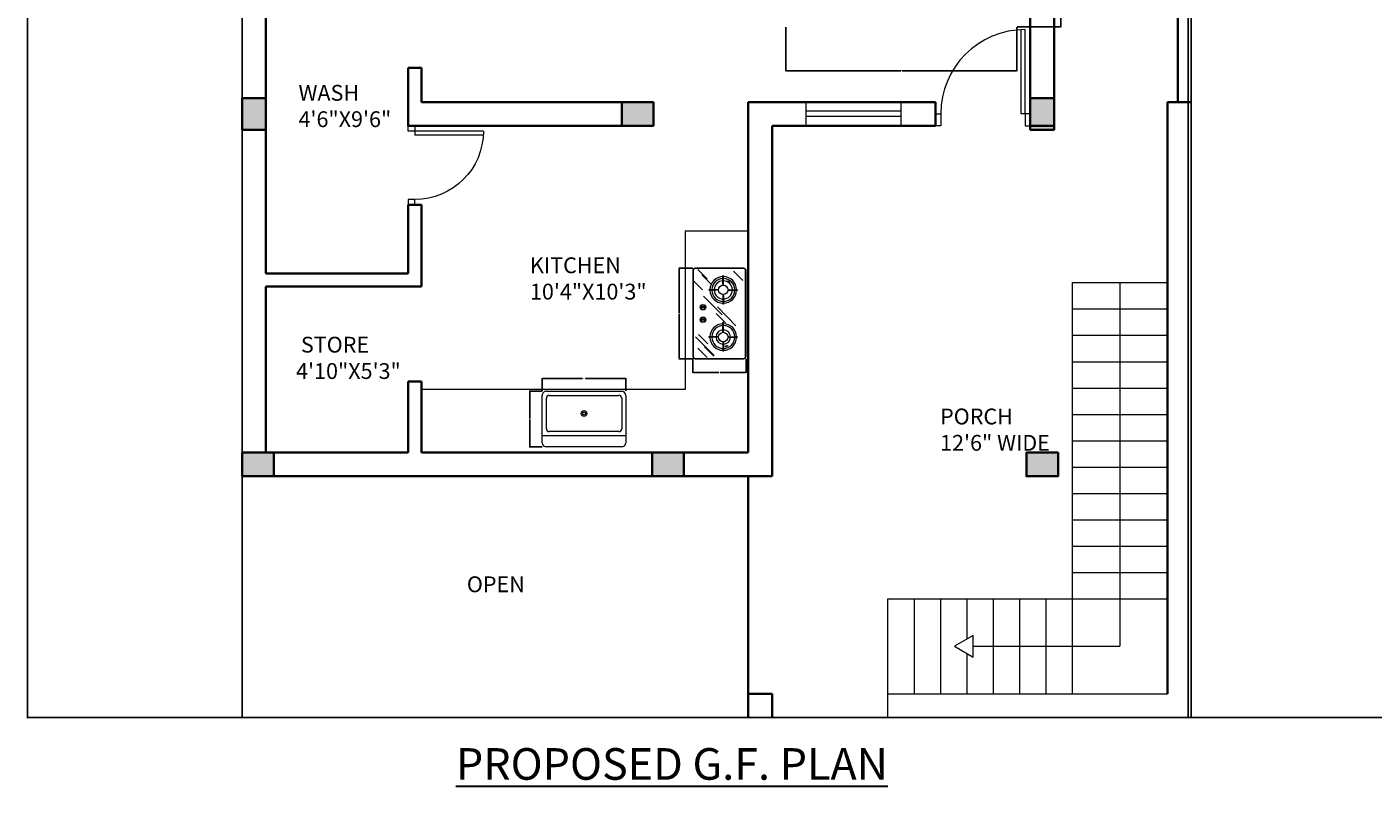
# Model space of a CAD drawing. Units: inches. Extents: x 1602 to 2642, y 1463 to 2270.
# Tile 1 of 5: x 1602 to 2113, y 1475 to 1763. Entities that reach past the tile are written whole.
import ezdxf

# ---------------------------------------------------------------- set-up
doc = ezdxf.new("R2010")
doc.units = ezdxf.units.IN
for name, color, linetype, lineweight in [('A-ANNO-DIMS', 2, 'Continuous', 18), ('A-ANNO-TEXT', 7, 'Continuous', 30), ('A-AREA-IDEN', 7, 'Continuous', 18), ('A-COLS', 7, 'Continuous', 35), ('A-DOOR', 3, 'Continuous', 18), ('A-EQPM', 8, 'Continuous', 18), ('A-FLOR-CASE', 9, 'Continuous', 18), ('A-FLOR-FIXT', 8, 'Continuous', 18), ('A-FLOR-STRS', 7, 'Continuous', 18), ('A-GLAZ', 4, 'Continuous', 18), ('A-WALL', 7, 'Continuous', 35), ('C-PROP', 7, 'Continuous', 25)]:
    doc.layers.add(name, color=color, linetype=linetype, lineweight=lineweight)
doc.styles.add('ATTR', font='romans.shx', dxfattribs={"width": 0.8, "height": 1.075})
doc.styles.get("Standard").update_dxf_attribs({"font": 'arial.ttf'})
doc.dimstyles.get("Standard").update_dxf_attribs({"dimtxt": 0.18, "dimasz": 0.18, "dimexe": 0.18, "dimexo": 0.0625, "dimgap": 0.09, "dimtad": 0, "dimtih": 1, "dimtoh": 1, "dimdec": 4, "dimzin": 0, "dimdsep": 46, "dimtxsty": 'Standard', "dimcen": 0.09, "dimadec": 0, "dimazin": 0, "dimtfac": 1, "dimtdec": 4, "dimtofl": 0, "dimtmove": 0, "dimatfit": 3, "dimfxl": 1, "dimtolj": 1, "dimtzin": 0, "dimarcsym": 0})

# ---------------------------------------------------------------- blocks, each defined once
blk = doc.blocks.new("30'' Sink Single PV")
blk.add_line((-15, -3.999996), (15, -3.999996))
for points in [[(-13.5, 0), (13.5, 0)], [(-15, -18.499996), (-15, -1.5)], [(15, -1.5), (15, -18.499996)], [(-13.5, -17.499996), (-13.5, -6.499996)], [(-12.5, -5.499996), (12.5, -5.499996)], [(13.5, -6.499996), (13.5, -17.499996)], [(12.5, -18.499996), (-12.5, -18.499996)], [(13.5, -19.999996), (-13.5, -19.999996)]]:
    blk.add_lwpolyline(points)
for radius in [1, 0.5]:
    blk.add_circle((0, -11.999996), radius)
for centre, radius, start, end in [((-13.5, -1.5), 1.5, 90, 180), ((13.5, -1.5), 1.5, 0, 90), ((-12.5, -6.499996), 1, 90, 180), ((12.5, -6.499996), 1, 0, 90), ((-13.5, -18.499996), 1.5, 180, 270), ((-12.5, -17.499996), 1, 180, 270), ((12.5, -17.499996), 1, 270, 0), ((13.5, -18.499996), 1.5, 270, 0)]:
    blk.add_arc(centre, radius, start, end)
at = {"style": 'ATTR', "width": 0.8, "flags": 9}
blk.add_attdef('ESTCODE', (0, 0), '', height=0.006, dxfattribs=at)
blk = doc.blocks.new('A$C525172BA')
for p, q in [((24, 337), (101, 414)), ((178, 369), (183, 369)), ((321, 203), (476, 357)), ((572, 369), (567, 369)), ((63, 254), (63, 249)), ((232, 89), (387, 244)), ((299, 254), (299, 249)), ((374, 194), (452, 271)), ((451, 254), (451, 249)), ((687, 254), (687, 249)), ((10, 41), (87, 118)), ((55, 74), (132, 151)), ((178, 133), (183, 133)), ((550, 48), (627, 125)), ((572, 133), (567, 133)), ((568, 22), (722, 177)), ((651, 97), (728, 175)), ((661, 42), (739, 119)), ((101, 2), (178, 79))]:
    blk.add_line(p, q)
at = {"ltscale": 0.18}
for p, q in [((178, 297), (178, 369)), ((183, 297), (183, 369)), ((567, 297), (567, 369)), ((572, 297), (572, 369)), ((135, 254), (63, 254)), ((135, 249), (63, 249)), ((225, 254), (299, 254)), ((225, 249), (299, 249)), ((525, 254), (451, 254)), ((525, 249), (451, 249)), ((615, 254), (687, 254)), ((615, 249), (687, 249)), ((178, 207), (178, 133)), ((183, 207), (183, 133)), ((567, 207), (567, 133)), ((572, 207), (572, 133)), ((319, 100), (319, 69)), ((327, 100), (327, 69)), ((423, 100), (423, 69)), ((431, 100), (431, 69))]:
    blk.add_line(p, q, dxfattribs=at)
for points in [[(20, 0), (730, 0, 0.414214), (750, 20), (750, 420, 0.414214), (730, 440), (20, 440, 0.414214), (0, 420), (0, 20, 0.414214)], [(20, 3), (730, 3, 0.414214), (747, 20), (747, 420, 0.414214), (730, 437), (20, 437, 0.414214), (3, 420), (3, 20, 0.414214)]]:
    blk.add_lwpolyline(points, format="xyb", close=True)
for centre in [(109, 291), (115, 300), (643, 284), (647, 273)]:
    blk.add_circle(centre, 3.58)
for centre, radius in [((180, 252), 39), ((570, 252), 39), ((323, 84), 22.5), ((427, 84), 22.5)]:
    blk.add_circle(centre, radius, dxfattribs=at)
for centre, radius, start, end in [((180, 252), 110, 91.3023, 178.6977), ((180, 252), 95, 91.5918, 178.4082), ((180, 252), 110, 1.3023, 88.6977), ((180, 252), 95, 1.5918, 88.4082), ((570, 252), 110, 91.3023, 178.6977), ((570, 252), 95, 91.5918, 178.4082), ((570, 252), 110, 1.3023, 88.6977), ((570, 252), 95, 1.5918, 88.4082), ((180, 252), 110, 181.3023, 268.6977), ((180, 252), 95, 181.5918, 268.4082), ((180, 252), 75, 91.9102, 178.0898), ((180, 252), 75, 181.9102, 268.0898), ((134, 252), 2.64, 288.751, 71.249), ((180, 297), 2.52, 186.7354, 353.2646), ((180, 252), 75, 1.9102, 88.0898), ((180, 252), 75, 271.9102, 358.0898), ((180, 252), 110, 271.3023, 358.6977), ((180, 252), 95, 271.5918, 358.4082), ((226, 252), 2.67, 110.5507, 249.4493), ((570, 252), 110, 181.3023, 268.6977), ((570, 252), 95, 181.5918, 268.4082), ((570, 252), 60, 92.388, 177.612), ((570, 252), 60, 182.388, 267.612), ((524, 252), 2.63, 288.412, 71.588), ((570, 297), 2.51, 183.9579, 356.0421), ((570, 252), 60, 2.388, 87.612), ((570, 252), 60, 272.388, 357.612), ((570, 252), 110, 271.3023, 358.6977), ((570, 252), 95, 271.5918, 358.4082), ((615, 252), 2.58, 104.2945, 255.7055), ((180, 206), 2.69, 21.7885, 158.2115), ((570, 206), 2.63, 17.9418, 162.0582), ((323, 84), 18.5, 111.3237, 248.6763), ((317, 100), 2, 0, 111.3237), ((317, 69), 2, 248.6763, 0), ((329, 100), 2, 68.6763, 180), ((329, 69), 2, 180, 291.3237), ((323, 84), 18.5, 291.3237, 68.6763), ((427, 84), 18.5, 111.3237, 248.6763), ((421, 100), 2, 0, 111.3237), ((421, 69), 2, 248.6763, 0), ((433, 100), 2, 68.6763, 180), ((433, 69), 2, 180, 291.3237), ((427, 84), 18.5, 291.3237, 68.6763)]:
    blk.add_arc(centre, radius, start, end, dxfattribs=at)
blk = doc.blocks.new('DOOR-SWING-26IN')
for p, q in [((26.5, 28.46), (26.5, 2.5)), ((28, 28.5), (28, 2.5)), ((0, 2.5), (2, 2.5)), ((2, 2.5), (2, 0)), ((28, 2.5), (26.5, 2.5)), ((30, 2.5), (28, 2.5)), ((28, 2.5), (28, 0)), ((2, 0), (0, 0)), ((28, 0), (30, 0))]:
    blk.add_line(p, q)
blk.add_arc((28, 2.5), 26, 90, 180)
blk = doc.blocks.new('DOOR-SWING-32IN')
for p, q in [((32.5, 4.5), (32.5, 36.46)), ((34, 4.5), (34, 36.5)), ((0, 4.5), (2, 4.5)), ((2, 0), (0, 0)), ((2, 4.5), (2, 0)), ((34, 4.5), (32.5, 4.5)), ((36, 4.5), (34, 4.5)), ((34, 4.5), (34, 0)), ((34, 0), (36, 0))]:
    blk.add_line(p, q)
blk.add_arc((34, 4.5), 32, 90, 180)
blk = doc.blocks.new('WIN-36IN')
for p, q in [((0, 0), (0, 9)), ((36, 5.5), (0, 5.5)), ((36, 0), (36, 9)), ((36, 3.5), (0, 3.5))]:
    blk.add_line(p, q)
blk = doc.blocks.new('COL-12X9')
h = blk.add_hatch(color=256)
h.dxf.hatch_style = 1
h.paths.add_polyline_path([(12, 0), (12, 9), (0, 9), (0, 0)])
blk.add_lwpolyline([(12, 9), (12, 0), (0, 0), (0, 9)], close=True)
blk = doc.blocks.new('STAIR-PORCH-RETURN')
for p, q in [((70, 9), (70, 165)), ((70, 165), (106, 165)), ((88, 165), (88, 27)), ((70, 155), (106, 155)), ((70, 145), (106, 145)), ((70, 135), (106, 135)), ((70, 125), (106, 125)), ((70, 115), (106, 115)), ((70, 105), (106, 105)), ((70, 95), (106, 95)), ((70, 85), (106, 85)), ((70, 75), (106, 75)), ((70, 65), (106, 65)), ((70, 55), (106, 55)), ((0, 45), (106, 45)), ((0, 0), (0, 45)), ((10, 9), (10, 45)), ((20, 9), (20, 45)), ((30, 29.72), (30, 45)), ((40, 9), (40, 45)), ((50, 9), (50, 45)), ((60, 9), (60, 45)), ((32.36, 27), (88, 27)), ((30, 9), (30, 24.28)), ((0, 9), (106, 9))]:
    blk.add_line(p, q)
blk.add_lwpolyline([(25.29, 27), (32.36, 22.92), (32.36, 31.08)], close=True)
blk = doc.blocks.new('*D19')
at = {"layer": 'A-ANNO-DIMS', "color": 0, "lineweight": -2, "transparency": 16777216}
for p, q in [((1977.68, 1873.68), (1994.44, 1873.68)), ((1994.26, 1873.5), (1994.26, 1818.41)), ((1994.26, 1762.95), (1994.26, 1818.04)), ((1977.68, 1762.77), (1994.44, 1762.77))]:
    blk.add_line(p, q, dxfattribs=at)
at = {"layer": 'A-ANNO-DIMS', "color": 0, "transparency": 16777216}
for points in [[(1994.23, 1873.5), (1994.29, 1873.5), (1994.26, 1873.68)], [(1994.23, 1762.95), (1994.29, 1762.95), (1994.26, 1762.77)]]:
    blk.add_solid(points, dxfattribs=at)
at = {"layer": 'Defpoints', "color": 0, "transparency": 16777216}
for p in [(1977.62, 1873.68), (1977.62, 1762.77), (1994.26, 1762.77)]:
    blk.add_point(p, dxfattribs=at)
at = {"layer": 'A-ANNO-DIMS', "color": 0, "transparency": 16777216, "insert": (1994.26, 1818.22), "char_height": 0.18, "attachment_point": 5}
blk.add_mtext('\\A1;SOFA SET 111', dxfattribs=at)
blk = doc.blocks.new('*D20')
at = {"layer": 'A-ANNO-DIMS', "color": 0, "lineweight": -2, "transparency": 16777216}
for p, q in [((1889.99, 1762.71), (1889.99, 1745.95)), ((1977.62, 1762.71), (1977.62, 1745.95)), ((1890.17, 1746.13), (1933.59, 1746.13)), ((1977.44, 1746.13), (1934.02, 1746.13))]:
    blk.add_line(p, q, dxfattribs=at)
at = {"layer": 'A-ANNO-DIMS', "color": 0, "transparency": 16777216}
for points in [[(1890.17, 1746.16), (1890.17, 1746.1), (1889.99, 1746.13)], [(1977.44, 1746.16), (1977.44, 1746.1), (1977.62, 1746.13)]]:
    blk.add_solid(points, dxfattribs=at)
at = {"layer": 'Defpoints', "color": 0, "transparency": 16777216}
for p in [(1889.99, 1762.77), (1977.62, 1762.77), (1889.99, 1746.13)]:
    blk.add_point(p, dxfattribs=at)
at = {"layer": 'A-ANNO-DIMS', "color": 0, "transparency": 16777216, "insert": (1933.81, 1746.13), "char_height": 0.18, "attachment_point": 5}
blk.add_mtext('\\A1;88', dxfattribs=at)
blk = doc.blocks.new('*D21')
at = {"layer": 'A-ANNO-DIMS', "color": 0, "lineweight": -2, "transparency": 16777216}
for p, q in [((1797.55, 1624.63), (1797.55, 1629.5)), ((1797.73, 1629.32), (1812.87, 1629.32)), ((1829.1, 1629.32), (1813.96, 1629.32)), ((1829.28, 1624.63), (1829.28, 1629.5))]:
    blk.add_line(p, q, dxfattribs=at)
at = {"layer": 'A-ANNO-DIMS', "color": 0, "transparency": 16777216}
for points in [[(1797.73, 1629.35), (1797.73, 1629.29), (1797.55, 1629.32)], [(1829.1, 1629.35), (1829.1, 1629.29), (1829.28, 1629.32)]]:
    blk.add_solid(points, dxfattribs=at)
at = {"layer": 'Defpoints', "color": 0, "transparency": 16777216}
for p in [(1797.55, 1629.32), (1797.55, 1624.56), (1829.28, 1624.56)]:
    blk.add_point(p, dxfattribs=at)
at = {"layer": 'A-ANNO-DIMS', "color": 0, "transparency": 16777216, "insert": (1813.42, 1629.32), "char_height": 0.18, "attachment_point": 5}
blk.add_mtext('\\A1;SINK 32', dxfattribs=at)
blk = doc.blocks.new('*D22')
at = {"layer": 'A-ANNO-DIMS', "color": 0, "lineweight": -2, "transparency": 16777216}
for p, q in [((1797.49, 1624.56), (1792.61, 1624.56)), ((1792.79, 1624.38), (1792.79, 1614.17)), ((1792.79, 1603.59), (1792.79, 1613.81)), ((1797.49, 1603.41), (1792.61, 1603.41))]:
    blk.add_line(p, q, dxfattribs=at)
at = {"layer": 'A-ANNO-DIMS', "color": 0, "transparency": 16777216}
for points in [[(1792.76, 1624.38), (1792.82, 1624.38), (1792.79, 1624.56)], [(1792.76, 1603.59), (1792.82, 1603.59), (1792.79, 1603.41)]]:
    blk.add_solid(points, dxfattribs=at)
at = {"layer": 'Defpoints', "color": 0, "transparency": 16777216}
for p in [(1797.55, 1624.56), (1792.79, 1603.41), (1797.55, 1603.41)]:
    blk.add_point(p, dxfattribs=at)
at = {"layer": 'A-ANNO-DIMS', "color": 0, "transparency": 16777216, "insert": (1792.79, 1613.99), "char_height": 0.18, "attachment_point": 5}
blk.add_mtext('\\A1;21', dxfattribs=at)
blk = doc.blocks.new('*D23')
at = {"layer": 'A-ANNO-DIMS', "color": 0, "lineweight": -2, "transparency": 16777216}
for p, q in [((1854.63, 1671.23), (1849.35, 1671.23)), ((1849.53, 1671.05), (1849.53, 1654.22)), ((1849.53, 1637.03), (1849.53, 1653.86)), ((1854.63, 1636.85), (1849.35, 1636.85))]:
    blk.add_line(p, q, dxfattribs=at)
at = {"layer": 'A-ANNO-DIMS', "color": 0, "transparency": 16777216}
for points in [[(1849.5, 1671.05), (1849.56, 1671.05), (1849.53, 1671.23)], [(1849.5, 1637.03), (1849.56, 1637.03), (1849.53, 1636.85)]]:
    blk.add_solid(points, dxfattribs=at)
at = {"layer": 'Defpoints', "color": 0, "transparency": 16777216}
for p in [(1854.69, 1671.23), (1849.53, 1636.85), (1854.69, 1636.85)]:
    blk.add_point(p, dxfattribs=at)
at = {"layer": 'A-ANNO-DIMS', "color": 0, "transparency": 16777216, "insert": (1849.53, 1654.04), "char_height": 0.18, "attachment_point": 5}
blk.add_mtext('\\A1;COOKTOP 34', dxfattribs=at)
blk = doc.blocks.new('*D24')
at = {"layer": 'A-ANNO-DIMS', "color": 0, "lineweight": -2, "transparency": 16777216}
for p, q in [((1854.69, 1636.79), (1854.69, 1631.51)), ((1874.87, 1636.79), (1874.87, 1631.51)), ((1854.87, 1631.69), (1864.56, 1631.69)), ((1874.69, 1631.69), (1865, 1631.69))]:
    blk.add_line(p, q, dxfattribs=at)
at = {"layer": 'A-ANNO-DIMS', "color": 0, "transparency": 16777216}
for points in [[(1854.87, 1631.72), (1854.87, 1631.66), (1854.69, 1631.69)], [(1874.69, 1631.72), (1874.69, 1631.66), (1874.87, 1631.69)]]:
    blk.add_solid(points, dxfattribs=at)
at = {"layer": 'Defpoints', "color": 0, "transparency": 16777216}
for p in [(1854.69, 1636.85), (1874.87, 1636.85), (1874.87, 1631.69)]:
    blk.add_point(p, dxfattribs=at)
at = {"layer": 'A-ANNO-DIMS', "color": 0, "transparency": 16777216, "insert": (1864.78, 1631.69), "char_height": 0.18, "attachment_point": 5}
blk.add_mtext('\\A1;20', dxfattribs=at)
blk = doc.blocks.new('*D40')
at = {"layer": 'A-ANNO-DIMS', "color": 0, "lineweight": -2, "transparency": 16777216}
for p, q in [((1683.66, 2100.75), (1602.08, 2100.75)), ((1602.26, 2100.57), (1602.26, 1800.93)), ((1602.26, 1500.93), (1602.26, 1800.57)), ((1683.66, 1500.75), (1602.08, 1500.75))]:
    blk.add_line(p, q, dxfattribs=at)
at = {"layer": 'A-ANNO-DIMS', "color": 0, "transparency": 16777216}
for points in [[(1602.23, 2100.57), (1602.29, 2100.57), (1602.26, 2100.75)], [(1602.23, 1500.93), (1602.29, 1500.93), (1602.26, 1500.75)]]:
    blk.add_solid(points, dxfattribs=at)
at = {"layer": 'Defpoints', "color": 0, "transparency": 16777216}
for p in [(1602.26, 2100.75), (1683.73, 2100.75), (1683.73, 1500.75)]:
    blk.add_point(p, dxfattribs=at)
at = {"layer": 'A-ANNO-DIMS', "color": 0, "transparency": 16777216, "insert": (1602.26, 1800.75), "char_height": 0.18, "attachment_point": 5}
blk.add_mtext('\\A1;600', dxfattribs=at)
blk = doc.blocks.new('*D42')
at = {"layer": 'A-ANNO-DIMS', "color": 0, "lineweight": -2, "transparency": 16777216}
for p, q in [((2130.59, 2100.75), (2042.46, 2100.75)), ((2042.64, 2100.57), (2042.64, 1800.93)), ((2042.64, 1500.93), (2042.64, 1800.57)), ((2130.59, 1500.75), (2042.46, 1500.75))]:
    blk.add_line(p, q, dxfattribs=at)
at = {"layer": 'A-ANNO-DIMS', "color": 0, "transparency": 16777216}
for points in [[(2042.61, 2100.57), (2042.67, 2100.57), (2042.64, 2100.75)], [(2042.61, 1500.93), (2042.67, 1500.93), (2042.64, 1500.75)]]:
    blk.add_solid(points, dxfattribs=at)
at = {"layer": 'Defpoints', "color": 0, "transparency": 16777216}
for p in [(2042.64, 2100.75), (2130.66, 2100.75), (2130.66, 1500.75)]:
    blk.add_point(p, dxfattribs=at)
at = {"layer": 'A-ANNO-DIMS', "color": 0, "transparency": 16777216, "insert": (2042.64, 1800.75), "char_height": 0.18, "attachment_point": 5}
blk.add_mtext('\\A1;600', dxfattribs=at)

msp = doc.modelspace()

# ---------------------------------------------------------------- linework, layer by layer
at = {"layer": 'A-FLOR-CASE'}
for p, q in [((1851.73, 1685.38), (1851.73, 1625.25)), ((1851.73, 1685.38), (1875.73, 1685.38)), ((1851.73, 1625.25), (1751.73, 1625.25))]:
    msp.add_line(p, q, dxfattribs=at)
at = {"layer": 'A-WALL'}
for p, q in [((2038.73, 1734.25), (2038.73, 2100.75)), ((1991.73, 2040.25), (1991.73, 1725.25)), ((1982.73, 1878.25), (1982.73, 1725.25)), ((1692.73, 1783.25), (1692.73, 1669.25)), ((1751.73, 1747.25), (1746.73, 1747.25)), ((1746.73, 1747.25), (1746.73, 1725.25)), ((1751.73, 1747.25), (1751.73, 1734.25)), ((1839.73, 1734.25), (1751.73, 1734.25)), ((1839.73, 1734.25), (1839.73, 1725.25)), ((1875.73, 1734.25), (1875.73, 1601.25)), ((1946.73, 1734.25), (1875.73, 1734.25)), ((1946.73, 1734.25), (1946.73, 1725.25)), ((2043.73, 1734.25), (2034.73, 1734.25)), ((2034.73, 1509.75), (2034.73, 1734.25)), ((1839.73, 1725.25), (1746.73, 1725.25)), ((1884.73, 1725.25), (1884.73, 1592.25)), ((1946.73, 1725.25), (1884.73, 1725.25)), ((1991.73, 1725.25), (1982.73, 1725.25)), ((1751.73, 1695.25), (1746.73, 1695.25)), ((1746.73, 1695.25), (1746.73, 1669.25)), ((1751.73, 1695.25), (1751.73, 1664.25)), ((1746.73, 1669.25), (1692.73, 1669.25)), ((1751.73, 1664.25), (1692.73, 1664.25)), ((1692.73, 1664.25), (1692.73, 1601.25)), ((1746.73, 1628.25), (1746.73, 1601.25)), ((1751.73, 1628.25), (1746.73, 1628.25)), ((1751.73, 1628.25), (1751.73, 1601.25)), ((1746.73, 1601.25), (1692.73, 1601.25)), ((1875.73, 1601.25), (1751.73, 1601.25)), ((1884.73, 1592.25), (1683.73, 1592.25)), ((1875.73, 1592.25), (1875.73, 1500.75)), ((1875.73, 1509.75), (1884.73, 1509.75)), ((1884.73, 1509.75), (1884.73, 1500.75))]:
    msp.add_line(p, q, dxfattribs=at)
at = {"layer": 'C-PROP'}
for p, q in [((1683.73, 2100.75), (1683.73, 1500.75)), ((2043.73, 1500.75), (2043.73, 2100.75)), ((1683.73, 1500.75), (2043.73, 1500.75))]:
    msp.add_line(p, q, dxfattribs=at)

# ---------------------------------------------------------------- block references
at = {"layer": 'A-COLS', "rotation": 89.9999999999953}
for p in [(1692.73, 1723.75), (1991.73, 1723.75)]:
    msp.add_blockref('COL-12X9', p, dxfattribs=at)
at = {"layer": 'A-COLS'}
for p in [(1827.73, 1725.25), (1683.73, 1592.25), (1839.23, 1592.25), (1981.23, 1592.25)]:
    msp.add_blockref('COL-12X9', p, dxfattribs=at)
at = {"layer": 'A-DOOR'}
msp.add_blockref('DOOR-SWING-32IN', (1946.73, 1725.25), dxfattribs=at)
at = {"layer": 'A-DOOR', "extrusion": (0, 0, -1), "zscale": -1, "rotation": 89.99999999999991}
msp.add_blockref('DOOR-SWING-26IN', (-1746.73, 1695.25), dxfattribs=at)
at = {"layer": 'A-EQPM', "xscale": 0.0458485968829068, "yscale": 0.0458485968829068, "zscale": 0.0458485968829068, "rotation": 270}
msp.add_blockref('A$C525172BA', (1854.69, 1671.23), dxfattribs=at)
at = {"layer": 'A-FLOR-FIXT', "xscale": 1.057456869721644, "yscale": 1.057456869721644, "zscale": 1.057456869721644, "rotation": 180}
msp.add_blockref("30'' Sink Single PV", (1813.42, 1603.41), dxfattribs=at)
at = {"layer": 'A-FLOR-STRS'}
msp.add_blockref('STAIR-PORCH-RETURN', (1928.73, 1500.75), dxfattribs=at)
at = {"layer": 'A-GLAZ'}
msp.add_blockref('WIN-36IN', (1897.73, 1725.25), dxfattribs=at)

# ---------------------------------------------------------------- texts
at = {"layer": 'A-ANNO-TEXT', "insert": (1764.82, 1489.11), "char_height": 12, "attachment_point": 1}
msp.add_mtext_dynamic_manual_height_columns('{\\LPROPOSED G.F. PLAN}', width=211.2872, gutter_width=12.5, heights=[0], dxfattribs=at)
at = {"layer": 'A-AREA-IDEN', "char_height": 6, "attachment_point": 1}
for s, insert in [('WASH\\P4\'6"X9\'6"', (1705.09, 1740.76)), ('KITCHEN\\P10\'4"X10\'3"', (1792.89, 1675.33)), (' STORE\\P4\'10"X5\'3"', (1704.17, 1645.2)), ('PORCH\\P12\'6" WIDE', (1948.49, 1617.96)), ('OPEN ', (1768.96, 1554.28))]:
    msp.add_mtext_dynamic_manual_height_columns(s, width=62.8553, gutter_width=12.5, heights=[0], dxfattribs=dict(at, insert=insert))

# ---------------------------------------------------------------- dimensions: what is measured, and where the dimension line sits
at = {"layer": 'A-ANNO-DIMS'}
for base, p1, p2, angle, picture, middle in [((1602.26, 2100.75), (1683.73, 1500.75), (1683.73, 2100.75), 90, '*D40', (1602.26, 1800.75)), ((2042.64, 2100.75), (2130.66, 1500.75), (2130.66, 2100.75), 90, '*D42', (2042.64, 1800.75)), ((1889.99, 1746.13), (1977.62, 1762.77), (1889.99, 1762.77), 180, '*D20', (1933.81, 1746.13)), ((1792.79, 1603.41), (1797.55, 1624.56), (1797.55, 1603.41), 270, '*D22', (1792.79, 1613.99))]:
    dim = msp.add_linear_dim(base=base, p1=p1, p2=p2, angle=angle, dimstyle='Standard', override={"dimdec": 0, "dimlfac": 1, "dimrnd": 0, "dimzin": 0, "dimdsep": 46, "dimlunit": 2}, dxfattribs=at)
    dim.commit()
    dim.dimension.update_dxf_attribs({"geometry": picture, "text_midpoint": middle})
for base, p1, p2, angle, text, picture, middle in [((1994.26, 1762.77), (1977.62, 1873.68), (1977.62, 1762.77), 270, 'SOFA SET <>', '*D19', (1994.26, 1818.22)), ((1849.53, 1636.85), (1854.69, 1671.23), (1854.69, 1636.85), 270, 'COOKTOP <>', '*D23', (1849.53, 1654.04)), ((1797.55, 1629.32), (1829.28, 1624.56), (1797.55, 1624.56), 180, 'SINK <>', '*D21', (1813.42, 1629.32))]:
    dim = msp.add_linear_dim(base=base, p1=p1, p2=p2, angle=angle, text=text, dimstyle='Standard', override={"dimdec": 0, "dimlfac": 1, "dimrnd": 0, "dimzin": 0, "dimdsep": 46, "dimlunit": 2}, dxfattribs=at)
    dim.commit()
    dim.dimension.update_dxf_attribs({"geometry": picture, "text_midpoint": middle})
dim = msp.add_linear_dim(base=(1874.87, 1631.69), p1=(1854.69, 1636.85), p2=(1874.87, 1636.85), dimstyle='Standard', override={"dimdec": 0, "dimlfac": 1, "dimrnd": 0, "dimzin": 0, "dimdsep": 46, "dimlunit": 2}, dxfattribs=at)
dim.commit()
dim.dimension.update_dxf_attribs({"geometry": '*D24', "text_midpoint": (1864.78, 1631.69)})

doc.saveas('drawing.dxf')
